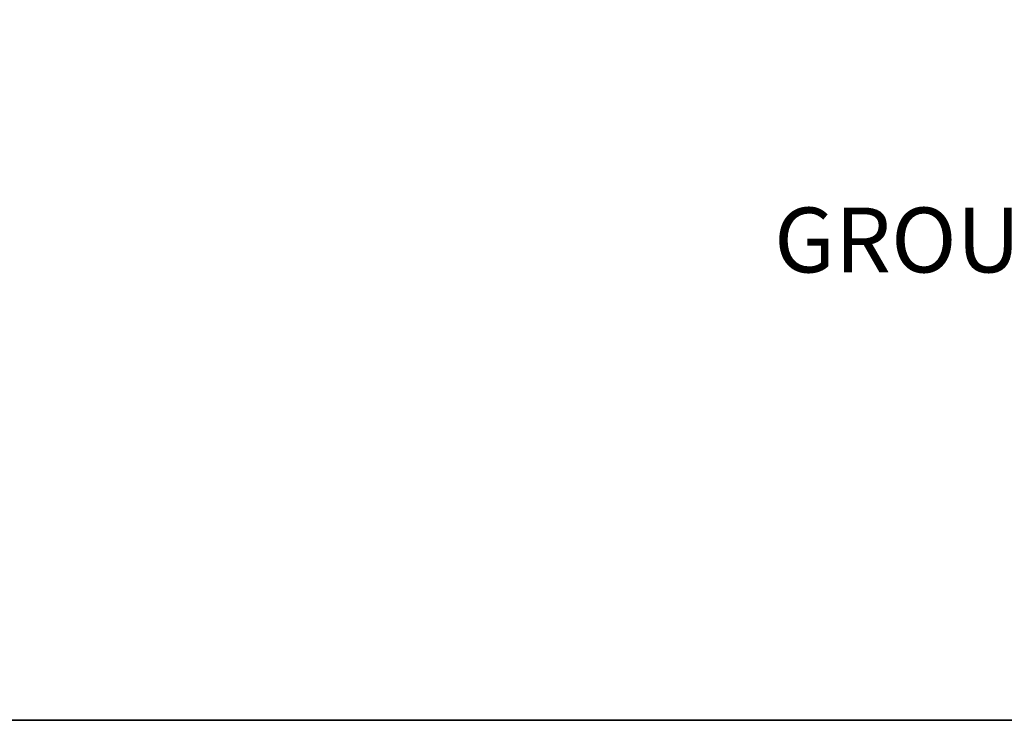
# Model space of a CAD drawing. Units: inches. Extents: x -31485 to -28799, y 18003 to 19130.
# Tile 1 of 15: x -31242 to -30999, y 18003 to 18176. Entities that reach past the tile are written whole.
import ezdxf

# ---------------------------------------------------------------- set-up
doc = ezdxf.new("R2010")
doc.units = ezdxf.units.IN
doc.layers.add('A-ANNO-TEXT', color=7, linetype='Continuous', lineweight=18)
doc.layers.add('A-ANNO-TTLB', color=7, linetype='Continuous', lineweight=35)
doc.styles.get("Standard").update_dxf_attribs({"font": 'arial.ttf'})

msp = doc.modelspace()

# ---------------------------------------------------------------- linework, layer by layer
at = {"layer": 'A-ANNO-TTLB'}
msp.add_lwpolyline([(-31485.09529421644, 19129.94040955191), (-28798.6381181599, 19129.94040955191), (-28798.6381181599, 18002.86338091846), (-31485.09529421644, 18002.86338091846)], close=True, dxfattribs=at)

# ---------------------------------------------------------------- texts
at = {"layer": 'A-ANNO-TEXT', "insert": (-31055.39833918592, 18129.45743188856), "char_height": 16, "attachment_point": 1}
msp.add_mtext_dynamic_manual_height_columns('{GROUND FLOOR PLAN}', width=1323.91503037831, gutter_width=12.5, heights=[0], dxfattribs=at)

doc.saveas('drawing.dxf')
